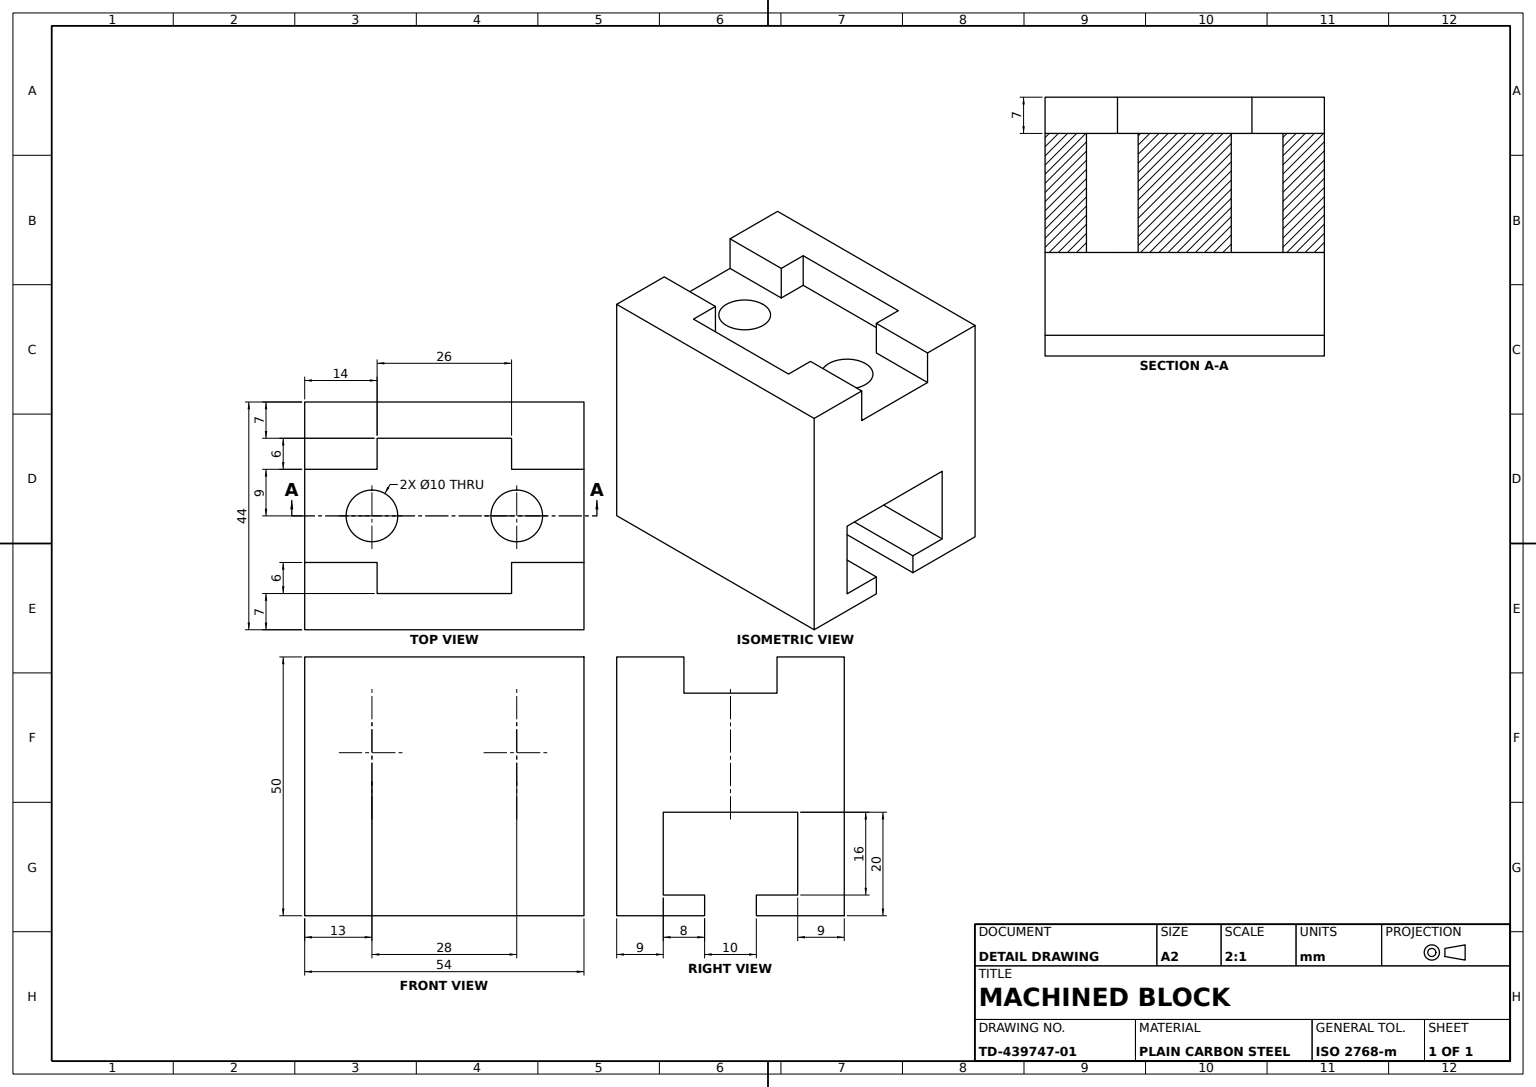
SolidWorks part; units mm, degrees
material "Plain Carbon Steel"
ref_plane "Front Plane" through (0, 0, 0) normal (0, 0, 1) x (1, 0, 0)
ref_plane "Top Plane" through (0, 0, 0) normal (0, 1, 0) x (1, 0, 0)
ref_plane "Right Plane" through (0, 0, 0) normal (1, 0, 0) x (0, 0, -1)
sketch "Base Block Sketch" plane through (0, 0, 0) normal (0, 0, 1) x (1, 0, 0)
  line L1 (-27, -25) -> (27, -25)
  line L2 (-27, -25) -> (-27, 25)
  line L3 (-27, 25) -> (27, 25)
  line L4 (27, -25) -> (27, 25)
  line L5 (-27, -25) -> (27, 25) construction
  line L6 (-27, 25) -> (27, -25) construction
  point P0 (0, 0)
  dimension "D1" = 54
  dimension "D2" = 50
extrude "Base Block 54x50x44" add sketch "Base Block Sketch" against normal blind 44
sketch "Top Pocket Sketch" plane through (0, 25, 0) normal (0, 1, 0) x (1, 0, 0)
  line L0 (-13, 37) -> (13, 37)
  line L1 (-27, 44) -> (-27, 0) construction
  line L2 (27, 44) -> (27, 0) construction
  line L3 (-27, 22) -> (27, 22) construction
  line L4 (-27, 31) -> (-13, 31)
  line L5 (13, 37) -> (13, 31)
  line L6 (-13, 37) -> (-13, 31)
  line L7 (13, 31) -> (27, 31)
  line L8 (27, 44) -> (-27, 44) construction
  line L9 (13, 13) -> (27, 13)
  line L10 (-13, 7) -> (-13, 13)
  line L11 (13, 7) -> (13, 13)
  line L12 (-27, 13) -> (-13, 13)
  line L13 (-13, 7) -> (13, 7)
  line L14 (-27, 31) -> (-27, 13)
  line L15 (27, 31) -> (27, 13)
  dimension "D1" = 26
  dimension "D2" = 6
  dimension "D3" = 6
  dimension "D4" = 14
  dimension "D5" = 7
extrude "Top Pocket 7 Deep" cut sketch "Top Pocket Sketch" against normal blind 7
sketch "T-Slot Sketch" plane through (-27, 0, 0) normal (-1, 0, 0) x (0, 0, 1)
  line L0 (-27, -25) -> (-27, -21)
  line L1 (-44, -25) -> (0, -25) construction
  line L2 (-27, -21) -> (-35, -21)
  line L3 (-35, -21) -> (-35, -5)
  line L4 (-35, -5) -> (-9, -5)
  line L5 (-9, -5) -> (-9, -21)
  line L6 (-9, -21) -> (-17, -21)
  line L7 (-17, -21) -> (-17, -25)
  line L8 (-17, -25) -> (-27, -25)
  line L9 (-44, 25) -> (-44, -25) construction
  dimension "D1" = 10
  dimension "D2" = 16
  dimension "D3" = 26
  dimension "D4" = 20
  dimension "D5" = 9
  dimension "D7" = 8
extrude "T-Slot Cut" cut sketch "T-Slot Sketch" against normal through all
sketch "Pocket Holes Sketch" plane through (0, 18, 0) normal (0, 1, 0) x (1, 0, 0)
  line L1 (-27, 13) -> (-13, 13) construction
  circle A0 centre (-14, 22) radius 5
  circle A1 centre (14, 22) radius 5
  dimension "D1" = 10
  dimension "D2" = 10
  dimension "D3" = 28
  dimension "D4" = 14
  dimension "D5" = 9
extrude "Pocket Holes 2xØ10" cut sketch "Pocket Holes Sketch" against normal through all
